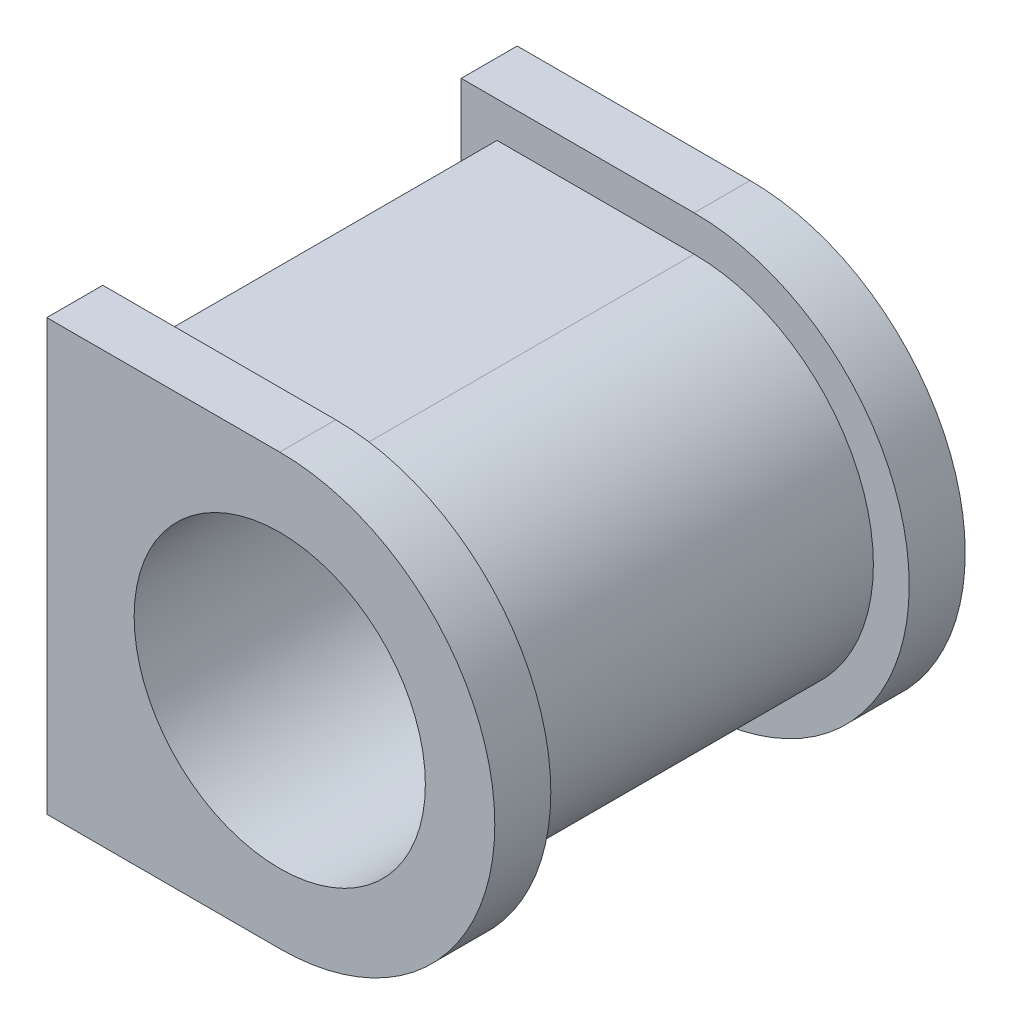
from build123d import *

# Parameters (mm, degrees)
BUSH_PROFILE_SKETCH_R   = 32.5
BUSH_BODY_DEPTH         = 40
FLANGE_PROFILE_SKETCH_R = 32.5
END_FLANGE_DEPTH        = 12.5


with BuildPart() as part:
    # Bush Profile Sketch → Bush Body (new, symmetric)
    with BuildSketch(Plane.XY):
        with BuildLine():
            Line((0, 40), (-44, 40))
            Line((-44, 40), (-44, -40))
            Line((-44, -40), (0, -40))
            ThreePointArc((0, -40), (40, 0), (0, 40))
        make_face()
        Circle(BUSH_PROFILE_SKETCH_R, mode=Mode.SUBTRACT)
    extrude(amount=BUSH_BODY_DEPTH, both=True)

    # Flange Profile Sketch → End Flange (add)
    with BuildSketch(Plane.XY.offset(40)):
        with BuildLine():
            Line((0, 48), (-52, 48))
            Line((-52, 48), (-52, -48))
            Line((-52, -48), (0, -48))
            ThreePointArc((0, -48), (48, 0), (0, 48))
        make_face()
        Circle(FLANGE_PROFILE_SKETCH_R, mode=Mode.SUBTRACT)
    end_flange = extrude(amount=END_FLANGE_DEPTH)

    # End Flange Mirror: End Flange across plane
    add(end_flange.mirror(Plane.XY))


solid = part.part
